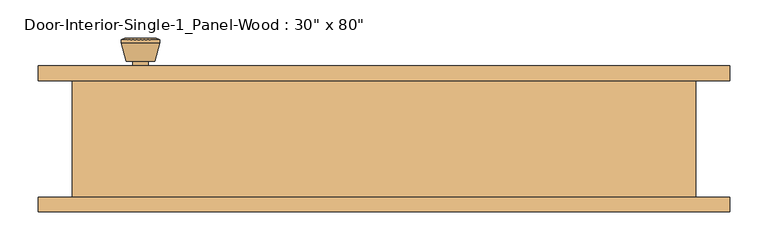
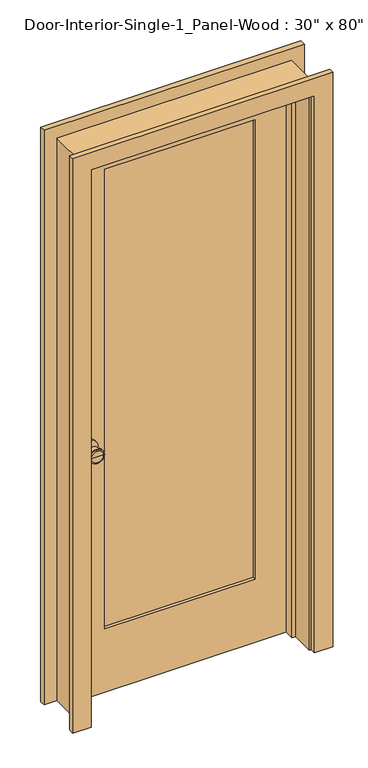
"""IFC4 building model written with IfcOpenShell, lengths in millimetres: door geometry."""

from ifc_helpers import new_model, si_unit, point, frame, frame_2d, origin, place, context, project, spatial, polyline, circle_curve, trimmed, segment, composite_curve, outline, extrude, faceted_brep, source, transform, mapped, element, save
from ifc_brep_helpers import plane_surface, cylinder_surface, revolved_surface, advanced_brep


def door_a1d926d7(model_context):
    return source(origin(), model_context, "Body", "SolidModel", [
        advanced_brep(
        [(-317.5, 32.1, 914.4), (-307.5, 32.1, 914.4), (-327.5, 32.1, 914.4), (-297.0241324, -16.9, 914.4), (-317.5, -16.9, 914.4), (-337.9758676, -16.9, 914.4), (-292.5, -15.0721319, 914.4), (-342.5, -15.0721319, 914.4), (-292.5, -11.6084537, 914.4), (-342.5, -11.6084537, 914.4), (-298.863764, 13.1, 914.4), (-336.136236, 13.1, 914.4), (-307.5, 13.1, 914.4), (-327.5, 13.1, 914.4)],
        [
            (0, 1),
            (1, 2, circle_curve(frame((-317.5, 32.1, 914.4), z_axis=(0.0, 1.0, 0.0), x_axis=(-1.0, 0.0, 0.0)), 10.0)),
            (2, 0),
            (2, 1, circle_curve(frame((-317.5, 32.1, 914.4), z_axis=(0.0, 1.0, 0.0), x_axis=(-1.0, 0.0, 0.0)), 10.0)),
            (3, 4),
            (4, 5),
            (5, 3, circle_curve(frame((-317.5, -16.9, 914.4), z_axis=(0.0, -1.0, 0.0), x_axis=(-1.0, 0.0, 0.0)), 20.4758676)),
            (3, 5, circle_curve(frame((-317.5, -16.9, 914.4), z_axis=(0.0, -1.0, 0.0), x_axis=(-1.0, 0.0, 0.0)), 20.4758676)),
            (6, 3),
            (5, 7),
            (7, 6, circle_curve(frame((-317.5, -15.0721319, 914.4), z_axis=(0.0, -1.0, 0.0), x_axis=(-1.0, 0.0, 0.0)), 25.0)),
            (6, 7, circle_curve(frame((-317.5, -15.0721319, 914.4), z_axis=(0.0, -1.0, 0.0), x_axis=(-1.0, 0.0, 0.0)), 25.0)),
            (8, 6),
            (7, 9),
            (9, 8, circle_curve(frame((-317.5, -11.6084537, 914.4), z_axis=(0.0, -1.0, 0.0), x_axis=(-1.0, 0.0, 0.0)), 25.0)),
            (8, 9, circle_curve(frame((-317.5, -11.6084537, 914.4), z_axis=(0.0, -1.0, 0.0), x_axis=(-1.0, 0.0, 0.0)), 25.0)),
            (10, 8),
            (9, 11),
            (11, 10, circle_curve(frame((-317.5, 13.1, 914.4), z_axis=(0.0, -1.0, 0.0), x_axis=(-1.0, 0.0, 0.0)), 18.636236)),
            (10, 11, circle_curve(frame((-317.5, 13.1, 914.4), z_axis=(0.0, -1.0, 0.0), x_axis=(-1.0, 0.0, 0.0)), 18.636236)),
            (12, 10),
            (11, 13),
            (13, 12, circle_curve(frame((-317.5, 13.1, 914.4), z_axis=(0.0, -1.0, 0.0), x_axis=(-1.0, 0.0, 0.0)), 10.0)),
            (12, 13, circle_curve(frame((-317.5, 13.1, 914.4), z_axis=(0.0, -1.0, 0.0), x_axis=(-1.0, 0.0, 0.0)), 10.0)),
            (1, 12),
            (13, 2),
        ],
        [
            plane_surface(frame((-317.5, 32.1, 914.4), z_axis=(0.0, 1.0, 0.0), x_axis=(-1.0, 0.0, 0.0))),
            plane_surface(frame((-317.5, -16.9, 914.4), z_axis=(0.0, -1.0, 0.0), x_axis=(-1.0, 0.0, 0.0))),
            revolved_surface(polyline([(-337.9758676, -16.9, 914.4), (-342.5, -15.0721319, 914.4)]), (-317.5, 32.1, 914.4), (0.0, 1.0, 0.0)),
            cylinder_surface(frame((-317.5, 32.1, 914.4), z_axis=(0.0, 1.0, 0.0), x_axis=(-1.0, 0.0, 0.0)), 25.0),
            revolved_surface(polyline([(-342.5, -11.6084537, 914.4), (-336.136236, 13.1, 914.4)]), (-317.5, 32.1, 914.4), (0.0, 1.0, 0.0)),
            plane_surface(frame((-317.5, 13.1, 914.4), z_axis=(0.0, 1.0, 0.0), x_axis=(-1.0, 0.0, 0.0))),
            cylinder_surface(frame((-317.5, 32.1, 914.4), z_axis=(0.0, 1.0, 0.0), x_axis=(-1.0, 0.0, 0.0)), 10.0),
        ],
        [
            (0, [[1, 2, 3]]),
            (0, [[-3, 4, -1]]),
            (1, [[5, 6, 7]]),
            (1, [[-6, -5, 8]]),
            (2, [[9, -7, 10, 11]]),
            (2, [[-10, -8, -9, 12]]),
            (3, [[13, -11, 14, 15]]),
            (3, [[-14, -12, -13, 16]]),
            (4, [[17, -15, 18, 19]]),
            (4, [[-18, -16, -17, 20]]),
            (5, [[21, -19, 22, 23]]),
            (5, [[-22, -20, -21, 24]]),
            (6, [[25, -23, 26, -2]]),
            (6, [[-26, -24, -25, -4]]),
        ],
    ),
        extrude(outline(composite_curve([segment(trimmed(circle_curve(frame_2d((914.4, -317.5)), 30.0), [point((914.4, -347.5))], [point((914.4, -287.5))], False, "CARTESIAN"), True, "CONTINUOUS"), segment(trimmed(circle_curve(frame_2d((914.4, -317.5)), 30.0), [point((914.4, -287.5))], [point((914.4, -347.5))], False, "CARTESIAN"), True, "CONTINUOUS")], self_intersect=False)), frame((0.0, 32.1, 0.0), z_axis=(0.0, 1.0, 0.0), x_axis=(0.0, 0.0, 1.0)), (0.0, 0.0, 1.0), 6.0),
        advanced_brep(
        [(-317.5, 79.025, 914.4), (-327.5, 79.025, 914.4), (-307.5, 79.025, 914.4), (-297.0241324, 128.025, 914.4), (-337.9758676, 128.025, 914.4), (-317.5, 128.025, 914.4), (-292.5, 126.1971319, 914.4), (-342.5, 126.1971319, 914.4), (-292.5, 122.7334537, 914.4), (-342.5, 122.7334537, 914.4), (-298.863764, 98.025, 914.4), (-336.136236, 98.025, 914.4), (-307.5, 98.025, 914.4), (-327.5, 98.025, 914.4)],
        [
            (0, 1),
            (1, 2, circle_curve(frame((-317.5, 79.025, 914.4), z_axis=(0.0, -1.0, 0.0), x_axis=(-1.0, 0.0, 0.0)), 10.0)),
            (2, 0),
            (2, 1, circle_curve(frame((-317.5, 79.025, 914.4), z_axis=(0.0, -1.0, 0.0), x_axis=(-1.0, 0.0, 0.0)), 10.0)),
            (3, 4, circle_curve(frame((-317.5, 128.025, 914.4), z_axis=(0.0, 1.0, 0.0), x_axis=(-1.0, 0.0, 0.0)), 20.4758676)),
            (4, 5),
            (5, 3),
            (4, 3, circle_curve(frame((-317.5, 128.025, 914.4), z_axis=(0.0, 1.0, 0.0), x_axis=(-1.0, 0.0, 0.0)), 20.4758676)),
            (6, 7, circle_curve(frame((-317.5, 126.1971319, 914.4), z_axis=(0.0, 1.0, 0.0), x_axis=(-1.0, 0.0, 0.0)), 25.0)),
            (7, 4),
            (3, 6),
            (7, 6, circle_curve(frame((-317.5, 126.1971319, 914.4), z_axis=(0.0, 1.0, 0.0), x_axis=(-1.0, 0.0, 0.0)), 25.0)),
            (8, 9, circle_curve(frame((-317.5, 122.7334537, 914.4), z_axis=(0.0, 1.0, 0.0), x_axis=(-1.0, 0.0, 0.0)), 25.0)),
            (9, 7),
            (6, 8),
            (9, 8, circle_curve(frame((-317.5, 122.7334537, 914.4), z_axis=(0.0, 1.0, 0.0), x_axis=(-1.0, 0.0, 0.0)), 25.0)),
            (10, 11, circle_curve(frame((-317.5, 98.025, 914.4), z_axis=(0.0, 1.0, 0.0), x_axis=(-1.0, 0.0, 0.0)), 18.636236)),
            (11, 9),
            (8, 10),
            (11, 10, circle_curve(frame((-317.5, 98.025, 914.4), z_axis=(0.0, 1.0, 0.0), x_axis=(-1.0, 0.0, 0.0)), 18.636236)),
            (12, 13, circle_curve(frame((-317.5, 98.025, 914.4), z_axis=(0.0, 1.0, 0.0), x_axis=(-1.0, 0.0, 0.0)), 10.0)),
            (13, 11),
            (10, 12),
            (13, 12, circle_curve(frame((-317.5, 98.025, 914.4), z_axis=(0.0, 1.0, 0.0), x_axis=(-1.0, 0.0, 0.0)), 10.0)),
            (1, 13),
            (12, 2),
        ],
        [
            plane_surface(frame((-317.5, 79.025, 914.4), z_axis=(0.0, -1.0, 0.0), x_axis=(-1.0, 0.0, 0.0))),
            plane_surface(frame((-317.5, 128.025, 914.4), z_axis=(0.0, 1.0, 0.0), x_axis=(-1.0, 0.0, 0.0))),
            revolved_surface(polyline([(-337.9758676, 128.025, 914.4), (-342.5, 126.1971319, 914.4)]), (-317.5, 79.025, 914.4), (0.0, -1.0, 0.0)),
            cylinder_surface(frame((-317.5, 79.025, 914.4), z_axis=(0.0, -1.0, 0.0), x_axis=(-1.0, 0.0, 0.0)), 25.0),
            revolved_surface(polyline([(-342.5, 122.7334537, 914.4), (-336.136236, 98.025, 914.4)]), (-317.5, 79.025, 914.4), (0.0, -1.0, 0.0)),
            plane_surface(frame((-317.5, 98.025, 914.4), z_axis=(0.0, -1.0, 0.0), x_axis=(-1.0, 0.0, 0.0))),
            cylinder_surface(frame((-317.5, 79.025, 914.4), z_axis=(0.0, -1.0, 0.0), x_axis=(-1.0, 0.0, 0.0)), 10.0),
        ],
        [
            (0, [[1, 2, 3]]),
            (0, [[-3, 4, -1]]),
            (1, [[5, 6, 7]]),
            (1, [[8, -7, -6]]),
            (2, [[9, 10, -5, 11]]),
            (2, [[12, -11, -8, -10]]),
            (3, [[13, 14, -9, 15]]),
            (3, [[16, -15, -12, -14]]),
            (4, [[17, 18, -13, 19]]),
            (4, [[20, -19, -16, -18]]),
            (5, [[21, 22, -17, 23]]),
            (5, [[24, -23, -20, -22]]),
            (6, [[-2, 25, -21, 26]]),
            (6, [[-4, -26, -24, -25]]),
        ],
    ),
        extrude(outline(composite_curve([segment(trimmed(circle_curve(frame_2d((914.4, -317.5)), 30.0), [point((914.4, -347.5))], [point((914.4, -287.5))], False, "CARTESIAN"), True, "CONTINUOUS"), segment(trimmed(circle_curve(frame_2d((914.4, -317.5)), 30.0), [point((914.4, -287.5))], [point((914.4, -347.5))], False, "CARTESIAN"), True, "CONTINUOUS")], self_intersect=False)), frame((0.0, 73.025, 0.0), z_axis=(0.0, 1.0, 0.0), x_axis=(0.0, 0.0, 1.0)), (0.0, 0.0, 1.0), 6.0),
        extrude(outline(polyline([(260.35, 49.7416667), (-260.35, 49.7416667), (-260.35, 61.3833333), (260.35, 61.3833333), (260.35, 49.7416667)])), frame((0.0, 0.0, 231.775), z_axis=(0.0, 0.0, 1.0), x_axis=(1.0, 0.0, 0.0)), (0.0, 0.0, 1.0), 1681.1625),
        extrude(outline(polyline([(2032.0, -381.0), (0.0, -381.0), (0.0, 381.0), (2032.0, 381.0), (2032.0, -381.0)]), holes=[polyline([(1912.9375, -260.35), (1912.9375, 260.35), (231.775, 260.35), (231.775, -260.35), (1912.9375, -260.35)])]), frame((0.0, 38.1, 0.0), z_axis=(0.0, 1.0, 0.0), x_axis=(0.0, 0.0, 1.0)), (0.0, 0.0, 1.0), 34.925),
        faceted_brep([(406.4, 73.025, 0.0), (406.4, -79.375, 0.0), (381.0, -79.375, 0.0), (381.0, 3.175, 0.0), (368.3, 3.175, 0.0), (368.3, 38.1, 0.0), (381.0, 38.1, 0.0), (381.0, 73.025, 0.0), (406.4, 73.025, 2057.4), (406.4, -79.375, 2057.4), (-406.4, -79.375, 2057.4), (-406.4, -79.375, 0.0), (-381.0, -79.375, 0.0), (-381.0, -79.375, 2032.0), (381.0, -79.375, 2032.0), (381.0, 3.175, 2032.0), (-381.0, 3.175, 2032.0), (-381.0, 3.175, 0.0), (-368.3, 3.175, 0.0), (-368.3, 3.175, 2019.3), (368.3, 3.175, 2019.3), (368.3, 38.1, 2019.3), (-368.3, 38.1, 2019.3), (-368.3, 38.1, 0.0), (-381.0, 38.1, 0.0), (-381.0, 38.1, 2032.0), (381.0, 38.1, 2032.0), (381.0, 73.025, 2032.0), (-381.0, 73.025, 2032.0), (-381.0, 73.025, 0.0), (-406.4, 73.025, 0.0), (-406.4, 73.025, 2057.4)], [[[0, 1, 2, 3, 4, 5, 6, 7]], [[1, 0, 8, 9]], [[2, 1, 9, 10, 11, 12, 13, 14]], [[3, 2, 14, 15]], [[4, 3, 15, 16, 17, 18, 19, 20]], [[5, 4, 20, 21]], [[6, 5, 21, 22, 23, 24, 25, 26]], [[7, 6, 26, 27]], [[0, 7, 27, 28, 29, 30, 31, 8]], [[9, 8, 31, 10]], [[15, 14, 13, 16]], [[21, 20, 19, 22]], [[27, 26, 25, 28]], [[30, 29, 24, 23, 18, 17, 12, 11]], [[10, 31, 30, 11]], [[16, 13, 12, 17]], [[22, 19, 18, 23]], [[28, 25, 24, 29]]]),
        extrude(outline(polyline([(0.0, 387.35), (0.0, 450.85), (2101.85, 450.85), (2101.85, -450.85), (0.0, -450.85), (0.0, -387.35), (2038.35, -387.35), (2038.35, 387.35), (0.0, 387.35)])), frame((0.0, -98.425, 0.0), z_axis=(0.0, 1.0, 0.0), x_axis=(0.0, 0.0, 1.0)), (0.0, 0.0, 1.0), 19.05),
        extrude(outline(polyline([(0.0, 387.35), (0.0, 450.85), (2101.85, 450.85), (2101.85, -450.85), (0.0, -450.85), (0.0, -387.35), (2038.35, -387.35), (2038.35, 387.35), (0.0, 387.35)])), frame((0.0, 73.025, 0.0), z_axis=(0.0, 1.0, 0.0), x_axis=(0.0, 0.0, 1.0)), (0.0, 0.0, 1.0), 19.05),
    ])


if __name__ == "__main__":
    model = new_model("IFC4")
    model_context = context("Model", 3, world=origin())
    ifc_project = project(units=[si_unit("LENGTHUNIT", "METRE", prefix="MILLI")], contexts=[model_context])
    site = spatial("IfcSite", under=ifc_project)
    building = spatial("IfcBuilding", under=site)
    placement = place(None, origin())
    door_shape = door_a1d926d7(model_context)
    element("IfcDoor", 1, ObjectType="Door-Interior-Single-1_Panel-Wood : 30\" x 80\"", at=placement, inside=building, context=model_context, shape_type="MappedRepresentation", body=[
        mapped(door_shape, transform((0.0, 0.0, 0.0), x_axis=(1.0, 0.0, 0.0), y_axis=(0.0, 1.0, 0.0), z_axis=(0.0, 0.0, 1.0))),
    ])
    save(model, "model.ifc")

# Revit data of these elements
# Type "Door-Interior-Single-1_Panel-Wood : 30\" x 80\""
#   Type Mark = "10"
#   Assembly Code = "C1020300"
#   Analytic Construction = "Wooden"
#   Top Rail = 0' - 4 11/16"
#   Thickness = 0' - 1 3/8"
#   Thermal Resistance (R) = 2.5876 (h·ft²·°F)/BTU
#   Swing Angle [instance default] = 90.00°
#   Stiles = 0' - 4 3/4"
#   Rough Width = 2' - 8"
#   Rough Height = 6' - 9"
#   Height = 6' - 8"
#   Width = 2' - 6"
#   Heat Transfer Coefficient (U) = 0.3865 BTU/(h·ft²·°F)
#   Bottom Rail = 0' - 9 1/8"
#   Trim Material = Cherry
#   Panel Material = Cherry
#   Frame Material = Cherry
#   Door Handle Material = Aluminum
#   Visual Light Transmittance = 0
#   Solar Heat Gain Coefficient = 0
#   Wall Closure = (empty or 0)
#   Function = (empty or 0)
# Element 1 (IfcDoor, "Door-Interior-Single-1_Panel-Wood : 30\" x 80\"")
#   Materials on its faces: "Cherry", "Aluminum"
# Materials
#   "Cherry": class "Wood", colour RGB 226 177 128, transparency 0, Description = "Prunus Serotina", Cost = 0
#   "Aluminum": class "Metal", colour RGB 247 247 247, transparency 0, Description = "Aluminum 6061", Cost = 0
